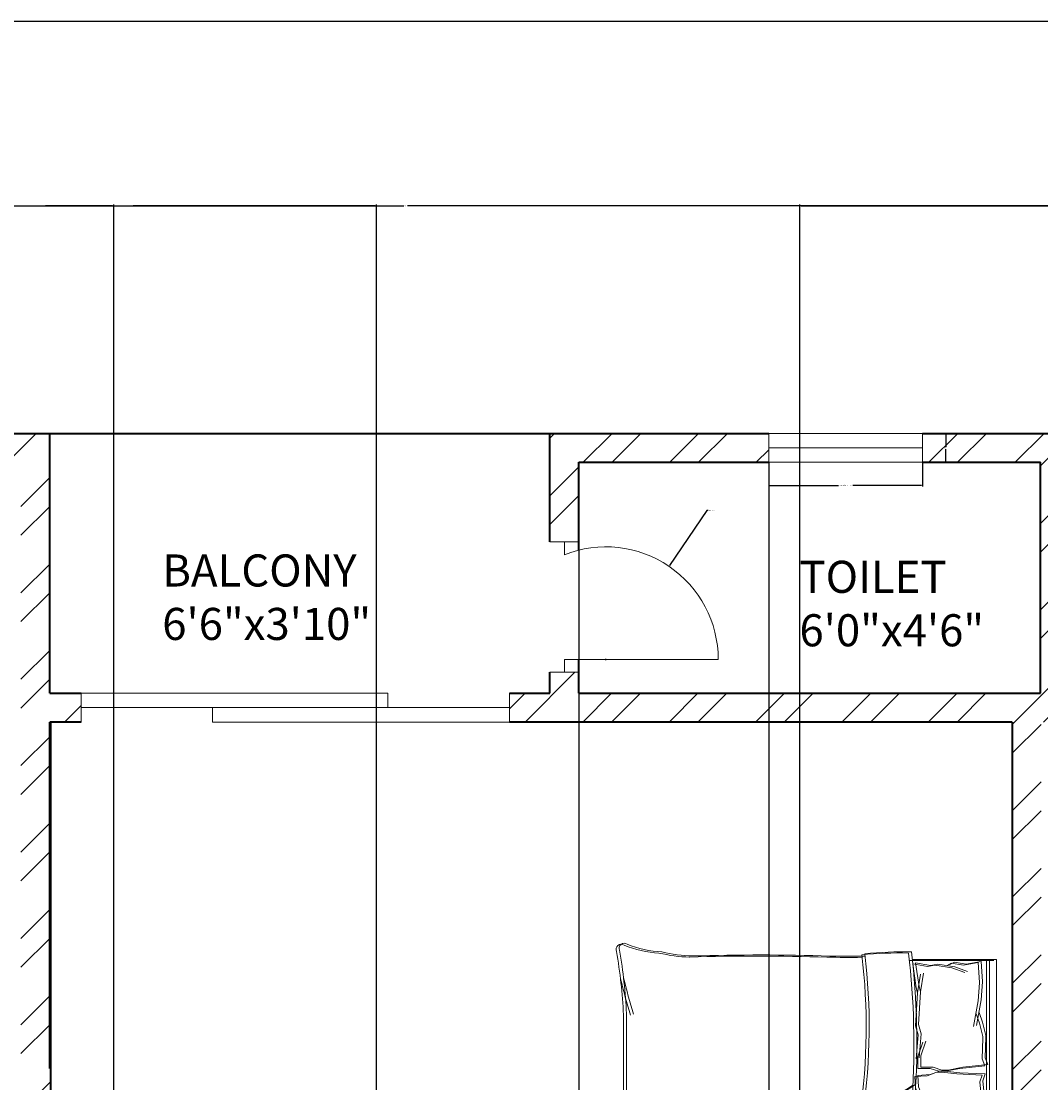
# Model space of a CAD drawing. Units: inches. Extents: x 2064 to 2782, y 1196 to 2299.
# Tile 8 of 11: x 2331 to 2490, y 2133 to 2299. Entities that reach past the tile are written whole.
import ezdxf

# ---------------------------------------------------------------- set-up
doc = ezdxf.new("R2010")
doc.units = ezdxf.units.IN
for name, color, linetype, lineweight in [('A-ANNO-DIMS', 2, 'Continuous', 18), ('A-ANNO-TTLB', 7, 'Continuous', 25), ('A-AREA-IDEN', 7, 'Continuous', 18), ('A-DOOR', 11, 'Continuous', 18), ('A-FURN', 8, 'Continuous', 13), ('A-GLAZ', 151, 'Continuous', 18), ('A-WALL', 7, 'Continuous', 35), ('A-WALL-PATT', 9, 'Continuous', 13)]:
    doc.layers.add(name, color=color, linetype=linetype, lineweight=lineweight)
doc.styles.get("Standard").update_dxf_attribs({"font": 'arial.ttf'})
doc.dimstyles.get("Standard").update_dxf_attribs({"dimtxt": 0.18, "dimasz": 0.18, "dimexe": 0.18, "dimexo": 0.0625, "dimgap": 0.09, "dimtad": 0, "dimtih": 1, "dimtoh": 1, "dimdec": 4, "dimzin": 0, "dimdsep": 46, "dimtxsty": 'Standard', "dimcen": 0.09, "dimadec": 0, "dimazin": 0, "dimtfac": 1, "dimtdec": 4, "dimtofl": 0, "dimtmove": 0, "dimatfit": 3, "dimfxl": 1, "dimtolj": 1, "dimtzin": 0, "dimarcsym": 0})

# ---------------------------------------------------------------- blocks, each defined once
blk = doc.blocks.new('BED-DOUBLE')
for p, q in [((2.53, 46.14), (2.53, 59.33)), ((2.53, 46.14), (2.53, 59.33)), ((2.53, 59.33), (37.35, 59.33)), ((2.53, 58.22), (37.35, 58.22)), ((2.53, 58.22), (37.35, 58.22)), ((2.7, 45.67), (2.7, 58.87)), ((2.7, 45.67), (2.7, 58.87)), ((17.88, 57.55), (18.93, 57.97)), ((17.88, 57.55), (18.93, 57.97)), ((18.93, 57.97), (19.35, 54.07)), ((18.93, 57.97), (19.35, 54.07)), ((37.35, 59.33), (37.35, 39.95)), ((37.35, 59.33), (37.35, 39.95)), ((37.52, 59.33), (37.52, 58.87)), ((37.52, 58.87), (37.52, 39.48)), ((37.52, 58.87), (37.52, 39.48)), ((2.7, 57.75), (37.52, 57.75)), ((2.7, 57.75), (37.52, 57.75)), ((2.84, 56.9), (5.96, 57.14)), ((2.84, 56.9), (5.96, 57.14)), ((2.84, 56.92), (3.26, 54.6)), ((2.84, 56.92), (3.26, 54.6)), ((3, 56.45), (3.43, 54.14)), ((3, 56.45), (3.43, 54.14)), ((3.01, 56.44), (6.13, 56.68)), ((3.01, 56.44), (6.13, 56.68)), ((5.96, 57.14), (6.04, 57.13)), ((5.96, 57.14), (6.04, 57.13)), ((6.04, 57.13), (8.82, 56.92)), ((6.04, 57.13), (8.82, 56.92)), ((6.13, 56.68), (6.2, 56.66)), ((6.13, 56.68), (6.2, 56.66)), ((6.2, 56.66), (8.99, 56.45)), ((6.2, 56.66), (8.99, 56.45)), ((8.82, 56.92), (12.82, 56.18)), ((8.82, 56.92), (12.82, 56.18)), ((8.99, 56.45), (12.99, 55.72)), ((8.99, 56.45), (12.99, 55.72)), ((10.82, 56.6), (12.3, 57.13)), ((10.82, 56.6), (12.3, 57.13)), ((10.99, 56.14), (12.46, 56.66)), ((10.99, 56.14), (12.46, 56.66)), ((12.3, 57.13), (14.4, 57.66)), ((12.3, 57.13), (14.4, 57.66)), ((12.46, 56.66), (14.57, 57.19)), ((12.46, 56.66), (14.57, 57.19)), ((14.4, 57.66), (14.64, 57.66)), ((14.4, 57.66), (14.64, 57.66)), ((14.57, 57.19), (14.8, 57.19)), ((14.57, 57.19), (14.8, 57.19)), ((14.64, 57.66), (17.88, 57.55)), ((14.64, 57.66), (17.88, 57.55)), ((14.8, 57.19), (18.04, 57.09)), ((14.8, 57.19), (18.04, 57.09)), ((18.04, 57.09), (19.1, 57.51)), ((18.04, 57.09), (19.1, 57.51)), ((19.1, 57.51), (19.52, 53.61)), ((19.1, 57.51), (19.52, 53.61)), ((20.38, 57.52), (20.2, 53.6)), ((20.38, 57.52), (20.21, 53.6)), ((20.55, 57.05), (20.37, 53.14)), ((20.55, 57.05), (20.37, 53.14)), ((21.46, 57.16), (20.38, 57.52)), ((21.46, 57.16), (20.38, 57.52)), ((21.63, 56.7), (20.55, 57.05)), ((21.63, 56.7), (20.55, 57.05)), ((24.69, 57.47), (21.46, 57.16)), ((24.69, 57.47), (21.46, 57.16)), ((24.85, 57.01), (21.63, 56.7)), ((24.85, 57.01), (21.63, 56.7)), ((24.92, 57.49), (24.69, 57.47)), ((24.92, 57.49), (24.69, 57.47)), ((25.09, 57.02), (24.85, 57.01)), ((25.09, 57.02), (24.85, 57.01)), ((27.05, 57.09), (24.92, 57.49)), ((27.05, 57.09), (24.92, 57.49)), ((27.22, 56.63), (25.09, 57.02)), ((27.22, 56.63), (25.09, 57.02)), ((30.54, 57.1), (26.59, 56.11)), ((30.54, 57.1), (26.59, 56.11)), ((30.7, 56.63), (26.75, 55.65)), ((30.7, 56.63), (26.75, 55.65)), ((28.56, 56.66), (27.05, 57.09)), ((28.56, 56.66), (27.05, 57.09)), ((28.73, 56.19), (27.22, 56.63)), ((28.73, 56.19), (27.22, 56.63)), ((33.3, 57.48), (30.54, 57.1)), ((33.3, 57.48), (30.54, 57.1)), ((33.47, 57.02), (30.7, 56.63)), ((33.47, 57.02), (30.7, 56.63)), ((36.51, 57.47), (32.57, 57.54)), ((32.57, 57.54), (33.3, 57.48)), ((36.51, 57.47), (32.57, 57.54)), ((32.57, 57.54), (33.3, 57.48)), ((36.68, 57.01), (32.74, 57.08)), ((32.74, 57.08), (33.47, 57.02)), ((36.67, 57.01), (32.74, 57.08)), ((32.74, 57.08), (33.47, 57.02)), ((36.51, 57.47), (36.23, 55.13)), ((36.51, 57.47), (36.23, 55.13)), ((36.68, 57.01), (36.4, 54.67)), ((36.67, 57.01), (36.4, 54.67)), ((3.68, 52.81), (4.42, 54.81)), ((3.68, 52.81), (4.42, 54.81)), ((35.92, 53.32), (35.06, 55.27)), ((35.92, 53.32), (35.06, 55.27)), ((36.09, 52.85), (35.23, 54.8)), ((36.09, 52.85), (35.23, 54.8)), ((36.23, 55.13), (36.67, 53.26)), ((36.23, 55.13), (36.67, 53.26)), ((36.4, 54.67), (36.83, 52.79)), ((36.4, 54.67), (36.83, 52.79)), ((3.26, 54.6), (2.94, 52.71)), ((3.26, 54.6), (2.94, 52.71)), ((3.43, 54.14), (3.11, 52.24)), ((3.43, 54.14), (3.11, 52.24)), ((3.85, 52.34), (4.58, 54.35)), ((3.85, 52.34), (4.58, 54.35)), ((19.35, 54.07), (19.77, 51.76)), ((19.35, 54.07), (19.77, 51.76)), ((19.52, 53.61), (19.94, 51.29)), ((19.52, 53.61), (19.94, 51.29)), ((20.21, 53.6), (19.93, 51.26)), ((20.2, 53.6), (19.93, 51.26)), ((20.37, 53.14), (20.1, 50.8)), ((20.37, 53.14), (20.1, 50.8)), ((36.51, 50.72), (35.92, 53.32)), ((36.51, 50.72), (35.92, 53.32)), ((36.67, 53.26), (36.29, 52.5)), ((36.67, 53.26), (36.29, 52.5)), ((2.94, 52.71), (3.36, 51.97)), ((2.94, 52.71), (3.36, 51.97)), ((3.11, 52.24), (3.53, 51.5)), ((3.11, 52.24), (3.53, 51.5)), ((3.26, 50.18), (3.68, 52.81)), ((3.26, 50.18), (3.68, 52.81)), ((3.43, 49.71), (3.85, 52.34)), ((3.43, 49.71), (3.85, 52.34)), ((19.77, 51.76), (19.77, 50.81)), ((19.77, 51.76), (19.77, 50.81)), ((36.68, 50.25), (36.09, 52.85)), ((36.67, 50.25), (36.09, 52.85)), ((36.83, 52.79), (36.46, 52.03)), ((36.83, 52.79), (36.46, 52.03)), ((3.47, 49.02), (3.26, 50.18)), ((3.47, 49.02), (3.26, 50.18)), ((3.64, 48.55), (3.43, 49.71)), ((3.64, 48.55), (3.43, 49.71)), ((19.77, 50.81), (19.35, 49.44)), ((19.77, 50.81), (19.35, 49.44)), ((19.94, 50.34), (19.52, 48.97)), ((19.94, 50.34), (19.52, 48.97)), ((19.93, 51.26), (19.99, 50.32)), ((19.93, 51.26), (19.99, 50.32)), ((19.94, 51.29), (19.94, 50.34)), ((19.94, 51.29), (19.94, 50.34)), ((19.99, 50.32), (20.49, 48.98)), ((19.99, 50.32), (20.49, 48.98)), ((20.1, 50.8), (20.15, 49.85)), ((20.1, 50.8), (20.15, 49.85)), ((20.15, 49.85), (20.66, 48.51)), ((20.15, 49.85), (20.66, 48.51)), ((36.37, 49.55), (36.51, 50.72)), ((36.37, 49.55), (36.51, 50.72)), ((36.54, 49.08), (36.68, 50.25)), ((36.54, 49.08), (36.67, 50.25)), ((3.05, 46.7), (3.47, 49.02)), ((3.05, 46.7), (3.47, 49.02)), ((3.21, 46.24), (3.64, 48.55)), ((3.21, 46.24), (3.64, 48.55)), ((17.56, 47.49), (15.27, 48.28)), ((17.56, 47.49), (15.27, 48.28)), ((19.35, 49.44), (19.35, 47.49)), ((19.35, 49.44), (19.35, 47.49)), ((19.52, 48.97), (19.52, 47.02)), ((19.52, 48.97), (19.52, 47.02)), ((20.49, 48.98), (20.62, 47.03)), ((20.49, 48.98), (20.62, 47.03)), ((20.66, 48.51), (20.78, 46.56)), ((20.66, 48.51), (20.78, 46.56)), ((22.4, 47.14), (24.64, 48.08)), ((22.4, 47.14), (24.64, 48.08)), ((36.94, 47.26), (36.37, 49.55)), ((36.94, 47.26), (36.37, 49.55)), ((37.1, 46.79), (36.54, 49.08)), ((37.1, 46.79), (36.54, 49.08)), ((6.76, 47.23), (3.05, 46.7)), ((6.76, 47.23), (3.05, 46.7)), ((6.93, 46.76), (3.21, 46.24)), ((6.93, 46.76), (3.21, 46.24)), ((4.65, 47.95), (7.59, 47.46)), ((4.65, 47.95), (7.59, 47.46)), ((4.82, 47.48), (7.75, 47)), ((4.82, 47.48), (7.75, 47)), ((7.59, 47.46), (6.76, 47.23)), ((7.59, 47.46), (6.76, 47.23)), ((7.75, 47), (6.93, 46.76)), ((7.75, 47), (6.93, 46.76)), ((7.59, 47.46), (12.69, 47.15)), ((7.59, 47.46), (12.69, 47.15)), ((7.75, 47), (12.86, 46.68)), ((7.75, 47), (12.86, 46.68)), ((12.69, 47.15), (14.12, 47.55)), ((12.69, 47.15), (14.12, 47.55)), ((12.86, 46.68), (14.29, 47.09)), ((12.86, 46.68), (14.29, 47.09)), ((14.12, 47.55), (17.86, 47.26)), ((14.12, 47.55), (17.86, 47.26)), ((14.29, 47.09), (18.03, 46.79)), ((14.29, 47.09), (18.03, 46.79)), ((17.73, 47.02), (15.44, 47.82)), ((17.73, 47.02), (15.44, 47.82)), ((19.35, 47.49), (17.56, 47.49)), ((19.35, 47.49), (17.56, 47.49)), ((19.52, 47.02), (17.73, 47.02)), ((19.52, 47.02), (17.73, 47.02)), ((20.62, 47.03), (22.4, 47.14)), ((20.62, 47.03), (22.4, 47.14)), ((20.78, 46.56), (22.57, 46.67)), ((20.78, 46.56), (22.57, 46.67)), ((22.05, 46.67), (25.1, 41.94)), ((22.05, 46.67), (25.1, 41.94)), ((22.57, 46.67), (24.81, 47.61)), ((22.57, 46.67), (24.81, 47.61)), ((29.61, 44.53), (23.54, 46.67)), ((29.61, 44.53), (23.54, 46.67)), ((23.72, 47.95), (26.66, 47.46)), ((23.72, 47.95), (26.66, 47.46)), ((23.89, 47.48), (26.83, 47)), ((23.89, 47.48), (26.83, 47)), ((26.66, 47.46), (31.77, 47.15)), ((26.66, 47.46), (31.77, 47.15)), ((26.83, 47), (31.94, 46.68)), ((26.83, 47), (31.94, 46.68)), ((31.77, 47.15), (33.2, 47.55)), ((31.77, 47.15), (33.2, 47.55)), ((31.94, 46.68), (33.36, 47.09)), ((31.94, 46.68), (33.36, 47.09)), ((33.2, 47.55), (36.94, 47.26)), ((33.2, 47.55), (36.94, 47.26)), ((33.36, 47.09), (37.1, 46.79)), ((33.36, 47.09), (37.1, 46.79)), ((22.21, 46.2), (25.26, 41.47)), ((22.21, 46.2), (25.26, 41.47)), ((29.78, 44.07), (23.7, 46.2)), ((29.78, 44.07), (23.7, 46.2)), ((33.67, 43.07), (29.61, 44.53)), ((33.67, 43.07), (29.61, 44.53)), ((33.84, 42.6), (29.78, 44.07)), ((33.84, 42.6), (29.78, 44.07)), ((35.82, 41.49), (33.67, 43.07)), ((35.82, 41.49), (33.67, 43.07)), ((25.1, 41.94), (26.34, 38.67)), ((25.1, 41.94), (26.34, 38.67)), ((25.26, 41.47), (26.51, 38.2)), ((25.26, 41.47), (26.51, 38.2)), ((35.98, 41.02), (33.84, 42.6)), ((35.98, 41.02), (33.84, 42.6)), ((38.52, 39.12), (35.82, 41.49)), ((38.52, 39.12), (35.82, 41.49)), ((38.68, 38.65), (35.98, 41.02)), ((38.68, 38.65), (35.98, 41.02)), ((26.34, 38.67), (26.56, 37.2)), ((26.34, 38.67), (26.56, 37.2)), ((26.51, 38.2), (26.73, 36.74)), ((26.51, 38.2), (26.73, 36.74)), ((28.37, 37.65), (29.84, 38.33)), ((28.37, 37.65), (29.84, 38.33)), ((29.84, 38.33), (32.32, 38.67)), ((29.84, 38.33), (32.32, 38.67)), ((30, 37.87), (32.49, 38.2)), ((30, 37.87), (32.49, 38.2)), ((32.32, 38.67), (35.14, 38.9)), ((32.32, 38.67), (35.14, 38.9)), ((32.49, 38.2), (35.31, 38.43)), ((32.49, 38.2), (35.31, 38.43)), ((35.14, 38.9), (37.4, 38.67)), ((35.14, 38.9), (37.4, 38.67)), ((35.31, 38.43), (37.56, 38.2)), ((35.31, 38.43), (37.56, 38.2)), ((37.4, 38.67), (38.52, 39.12)), ((37.4, 38.67), (38.52, 39.12)), ((37.56, 38.2), (38.68, 38.65)), ((37.56, 38.2), (38.68, 38.65)), ((38.57, 37.85), (38.52, 39.12, 2.82)), ((38.57, 37.85), (38.52, 39.12, 2.82)), ((38.74, 37.38), (38.68, 38.65, 2.82)), ((38.74, 37.38), (38.68, 38.65, 2.82)), ((26.56, 37.2), (28.37, 37.65)), ((26.56, 37.2), (28.37, 37.65)), ((26.73, 36.74), (28.54, 37.19)), ((26.73, 36.74), (28.54, 37.19)), ((28.54, 37.19), (30, 37.87)), ((28.54, 37.19), (30, 37.87)), ((10.97, 1.6), (28.91, 1.6)), ((10.97, 1.6), (28.91, 1.6)), ((11.14, 1.14), (29.07, 1.14)), ((11.14, 1.14), (29.07, 1.14))]:
    blk.add_line(p, q)
for centre, radius, start, end in [((15.56, -73.3), 120.19, 86.0865, 96.7821), ((15.56, -73.3), 120.19, 86.0865, 96.7821), ((15.73, -73.76), 120.19, 86.0865, 96.7821), ((15.73, -73.76), 120.19, 86.0865, 96.7821), ((62.04, 44.69), 60.69, 178.7218, 185.604), ((62.04, 44.69), 60.69, 178.7218, 185.604), ((62.21, 44.23), 60.69, 178.7218, 185.604), ((62.21, 44.23), 60.69, 178.7218, 185.604), ((12.94, -54.55), 94, 81.7845, 96.9006), ((12.94, -54.55), 94, 81.7845, 96.9006), ((13.1, -55.01), 94, 81.7845, 96.9006), ((13.1, -55.01), 94, 81.7845, 96.9006), ((-121.89, 36.62), 123.93, 358.4762, 1.0082), ((-121.89, 36.62), 123.93, 358.4762, 1.0082), ((-121.72, 36.16), 123.93, 358.4762, 1.0082), ((-121.72, 36.16), 123.93, 358.4762, 1.0082), ((31.87, 33.79), 4.53, 78.6608, 113.7384), ((31.87, 33.79), 4.53, 78.6608, 113.7384), ((37.39, 64.18), 26.36, 259.8763, 272.5657), ((37.39, 64.18), 26.36, 259.8763, 272.5657), ((26.69, 37.16), 0.134, 160.2464, 271.1377), ((26.69, 37.16), 0.134, 160.2464, 271.1377), ((22.7, 58.25), 21.6, 280.6617, 289.8806), ((22.7, 58.25), 21.6, 280.6617, 289.8806), ((26.86, 36.69), 0.134, 160.2464, 271.1377), ((26.86, 36.69), 0.134, 160.2464, 271.1377), ((22.86, 57.79), 21.6, 280.6617, 289.8806), ((22.86, 57.79), 21.6, 280.6617, 289.8806), ((32.04, 33.32), 4.53, 78.6608, 113.7384), ((32.04, 33.32), 4.53, 78.6608, 113.7384), ((37.56, 63.72), 26.36, 259.8763, 272.5657), ((37.56, 63.72), 26.36, 259.8763, 272.5657), ((132.79, 32.88), 94.35, 176.9791, 183.8365), ((132.79, 32.88), 94.35, 176.9791, 183.8365), ((132.95, 32.41), 94.35, 176.9791, 183.8365), ((132.95, 32.41), 94.35, 176.9791, 183.8365), ((353.21, 22.46), 351.38, 178.2277, 181.7185), ((353.21, 22.46), 351.38, 178.2277, 181.7185), ((353.38, 21.99), 351.38, 178.2277, 181.7185), ((353.38, 21.99), 351.38, 178.2277, 181.7185), ((-3284.8, 9.92), 3323.5, 0.00217, 0.28689), ((-3284.8, 9.92), 3323.5, 0.00217, 0.28689), ((-3284.64, 9.46), 3323.5, 0.00217, 0.28689), ((-3284.64, 9.46), 3323.5, 0.00217, 0.28689), ((-19.6, 12.33), 21.59, 346.0648, 358.9113), ((-19.6, 12.33), 21.59, 346.0648, 358.9113), ((-19.43, 11.87), 21.59, 346.0648, 358.9113), ((-19.43, 11.87), 21.59, 346.0648, 358.9113), ((55.48, 9.31), 16.8, 177.4714, 206.4681), ((55.48, 9.31), 16.8, 177.4714, 206.4681), ((55.65, 8.84), 16.8, 177.4714, 206.4681), ((55.65, 8.84), 16.8, 177.4714, 206.4681), ((-15.78, 8.14), 17.17, 337.9751, 356.652), ((-15.78, 8.14), 17.17, 337.9751, 356.652), ((-15.61, 7.67), 17.17, 337.9751, 356.652), ((-15.61, 7.67), 17.17, 337.9751, 356.652), ((0.79, 1.26), 0.793, 146.1736, 293.4781), ((0.79, 1.26), 0.793, 146.1736, 293.4781), ((-12.55, 76.61), 77.56, 283.3832, 287.7053), ((-12.55, 76.61), 77.56, 283.3832, 287.7053), ((-12.38, 76.14), 77.56, 283.3832, 287.7053), ((-12.38, 76.14), 77.56, 283.3832, 287.7053), ((39.64, 1.87), 0.803, 242.6588, 356.02), ((39.64, 1.87), 0.803, 242.6588, 356.02), ((0.96, 0.79), 0.793, 146.1736, 293.4781), ((0.96, 0.79), 0.793, 146.1736, 293.4781), ((15.61, -86.98), 88.71, 92.9958, 99.4091), ((15.61, -86.98), 88.71, 92.9958, 99.4091), ((15.78, -87.45), 88.71, 92.9958, 99.4091), ((15.78, -87.45), 88.71, 92.9958, 99.4091), ((29.98, -95.32), 96.92, 84.4998, 90.6351), ((29.98, -95.32), 96.92, 84.4998, 90.6351), ((30.15, -95.78), 96.92, 84.4998, 90.6351), ((30.15, -95.78), 96.92, 84.4998, 90.6351), ((39.81, 1.41), 0.803, 242.6588, 356.02), ((39.81, 1.41), 0.803, 242.6588, 356.02)]:
    blk.add_arc(centre, radius, start, end)
blk = doc.blocks.new('WIN-24IN')
for p, q in [((0, 0), (0, 4.5)), ((0, 4.5), (0, 2.25)), ((0, 4.5), (24, 4.5)), ((24, 2.25), (24, 4.5)), ((24, 4.5), (24, 0)), ((0, 2.25), (24, 2.25)), ((24, 0), (0, 0))]:
    blk.add_line(p, q)
blk = doc.blocks.new('*D14')
at = {"layer": 'A-ANNO-DIMS', "color": 0, "lineweight": -2, "transparency": 16777216}
for p, q in [((2447.29, 2229.73), (2447.29, 2226.01)), ((2471.29, 2229.73), (2471.29, 2226.01)), ((2447.47, 2226.19), (2458.17, 2226.19)), ((2471.11, 2226.19), (2460.41, 2226.19))]:
    blk.add_line(p, q, dxfattribs=at)
at = {"layer": 'A-ANNO-DIMS', "color": 0, "transparency": 16777216}
for points in [[(2447.47, 2226.22), (2447.47, 2226.16), (2447.29, 2226.19)], [(2471.11, 2226.22), (2471.11, 2226.16), (2471.29, 2226.19)]]:
    blk.add_solid(points, dxfattribs=at)
at = {"layer": 'Defpoints', "color": 0, "transparency": 16777216}
for p in [(2447.29, 2229.79), (2471.29, 2229.79), (2471.29, 2226.19)]:
    blk.add_point(p, dxfattribs=at)
at = {"layer": 'A-ANNO-DIMS', "color": 0, "transparency": 16777216, "insert": (2459.29, 2226.19), "char_height": 0.18, "attachment_point": 5}
blk.add_mtext('\\A1;WINDOW 24 TYP.', dxfattribs=at)
blk = doc.blocks.new('*D15')
at = {"layer": 'A-ANNO-DIMS', "color": 0, "lineweight": -2, "transparency": 16777216}
for p, q in [((2471.35, 2234.29), (2475.07, 2234.29)), ((2474.89, 2234.11), (2474.89, 2232.22)), ((2474.89, 2229.97), (2474.89, 2231.86)), ((2471.35, 2229.79), (2475.07, 2229.79))]:
    blk.add_line(p, q, dxfattribs=at)
at = {"layer": 'A-ANNO-DIMS', "color": 0, "transparency": 16777216}
for points in [[(2474.86, 2234.11), (2474.92, 2234.11), (2474.89, 2234.29)], [(2474.86, 2229.97), (2474.92, 2229.97), (2474.89, 2229.79)]]:
    blk.add_solid(points, dxfattribs=at)
at = {"layer": 'Defpoints', "color": 0, "transparency": 16777216}
for p in [(2471.29, 2234.29), (2474.89, 2234.29), (2471.29, 2229.79)]:
    blk.add_point(p, dxfattribs=at)
at = {"layer": 'A-ANNO-DIMS', "color": 0, "transparency": 16777216, "insert": (2474.89, 2232.04), "char_height": 0.18, "attachment_point": 5}
blk.add_mtext('\\A1;5 TYP.', dxfattribs=at)
blk = doc.blocks.new('*D22')
at = {"layer": 'A-ANNO-DIMS', "color": 0, "lineweight": -2, "transparency": 16777216}
for p, q in [((2128.17, 2234.35), (2128.17, 2269.97)), ((2128.35, 2269.79), (2390.38, 2269.79)), ((2652.99, 2269.79), (2390.96, 2269.79)), ((2653.17, 2234.35), (2653.17, 2269.97))]:
    blk.add_line(p, q, dxfattribs=at)
at = {"layer": 'A-ANNO-DIMS', "color": 0, "transparency": 16777216}
for points in [[(2128.35, 2269.82), (2128.35, 2269.76), (2128.17, 2269.79)], [(2652.99, 2269.82), (2652.99, 2269.76), (2653.17, 2269.79)]]:
    blk.add_solid(points, dxfattribs=at)
at = {"layer": 'Defpoints', "color": 0, "transparency": 16777216}
for p in [(2653.17, 2269.79), (2128.17, 2234.29), (2653.17, 2234.29)]:
    blk.add_point(p, dxfattribs=at)
at = {"layer": 'A-ANNO-DIMS', "color": 0, "transparency": 16777216, "insert": (2390.67, 2269.79), "char_height": 0.18, "attachment_point": 5}
blk.add_mtext('\\A1;525', dxfattribs=at)
blk = doc.blocks.new('*D23')
at = {"layer": 'A-ANNO-DIMS', "color": 0, "lineweight": -2, "transparency": 16777216}
for p, q in [((2653.23, 2234.29), (2688.85, 2234.29)), ((2688.67, 2234.11), (2688.67, 1937.72)), ((2688.67, 1640.97), (2688.67, 1937.36)), ((2452.23, 1640.79), (2688.85, 1640.79))]:
    blk.add_line(p, q, dxfattribs=at)
at = {"layer": 'A-ANNO-DIMS', "color": 0, "transparency": 16777216}
for points in [[(2688.64, 2234.11), (2688.7, 2234.11), (2688.67, 2234.29)], [(2688.64, 1640.97), (2688.7, 1640.97), (2688.67, 1640.79)]]:
    blk.add_solid(points, dxfattribs=at)
at = {"layer": 'Defpoints', "color": 0, "transparency": 16777216}
for p in [(2653.17, 2234.29), (2688.67, 2234.29), (2452.17, 1640.79)]:
    blk.add_point(p, dxfattribs=at)
at = {"layer": 'A-ANNO-DIMS', "color": 0, "transparency": 16777216, "insert": (2688.67, 1937.54), "char_height": 0.18, "attachment_point": 5}
blk.add_mtext('\\A1;593.5', dxfattribs=at)
blk = doc.blocks.new('*D27')
at = {"layer": 'A-ANNO-DIMS', "color": 0, "lineweight": -2, "transparency": 16777216}
for p, q in [((2452.17, 1640.85), (2452.17, 2269.97)), ((2452.35, 2269.79), (2493.09, 2269.79)), ((2534.61, 2269.79), (2493.87, 2269.79)), ((2534.79, 1643.35), (2534.79, 2269.97))]:
    blk.add_line(p, q, dxfattribs=at)
at = {"layer": 'A-ANNO-DIMS', "color": 0, "transparency": 16777216}
for points in [[(2452.35, 2269.82), (2452.35, 2269.76), (2452.17, 2269.79)], [(2534.61, 2269.82), (2534.61, 2269.76), (2534.79, 2269.79)]]:
    blk.add_solid(points, dxfattribs=at)
at = {"layer": 'Defpoints', "color": 0, "transparency": 16777216}
for p in [(2534.79, 2269.79), (2534.79, 1643.29), (2452.17, 1640.79)]:
    blk.add_point(p, dxfattribs=at)
at = {"layer": 'A-ANNO-DIMS', "color": 0, "transparency": 16777216, "insert": (2493.48, 2269.79), "char_height": 0.18, "attachment_point": 5}
blk.add_mtext('\\A1;82.62', dxfattribs=at)
blk = doc.blocks.new('*D35')
at = {"layer": 'A-ANNO-DIMS', "color": 0, "lineweight": -2, "transparency": 16777216}
for p, q in [((2309.4, 1932.85), (2309.4, 2269.97)), ((2309.58, 2269.79), (2347.37, 2269.79)), ((2385.94, 2269.79), (2348.16, 2269.79)), ((2386.12, 1856.35), (2386.12, 2269.97))]:
    blk.add_line(p, q, dxfattribs=at)
at = {"layer": 'A-ANNO-DIMS', "color": 0, "transparency": 16777216}
for points in [[(2309.58, 2269.82), (2309.58, 2269.76), (2309.4, 2269.79)], [(2385.94, 2269.82), (2385.94, 2269.76), (2386.12, 2269.79)]]:
    blk.add_solid(points, dxfattribs=at)
at = {"layer": 'Defpoints', "color": 0, "transparency": 16777216}
for p in [(2386.12, 2269.79), (2309.4, 1932.79), (2386.12, 1856.29)]:
    blk.add_point(p, dxfattribs=at)
at = {"layer": 'A-ANNO-DIMS', "color": 0, "transparency": 16777216, "insert": (2347.76, 2269.79), "char_height": 0.18, "attachment_point": 5}
blk.add_mtext('\\A1;76.72', dxfattribs=at)
blk = doc.blocks.new('*D39')
at = {"layer": 'A-ANNO-DIMS', "color": 0, "lineweight": -2, "transparency": 16777216}
for p, q in [((2322.95, 1645.35), (2322.95, 2269.97)), ((2323.13, 2269.79), (2333.59, 2269.79)), ((2344.97, 2269.79), (2334.51, 2269.79)), ((2345.15, 1645.35), (2345.15, 2269.97))]:
    blk.add_line(p, q, dxfattribs=at)
at = {"layer": 'A-ANNO-DIMS', "color": 0, "transparency": 16777216}
for points in [[(2323.13, 2269.82), (2323.13, 2269.76), (2322.95, 2269.79)], [(2344.97, 2269.82), (2344.97, 2269.76), (2345.15, 2269.79)]]:
    blk.add_solid(points, dxfattribs=at)
at = {"layer": 'Defpoints', "color": 0, "transparency": 16777216}
for p in [(2345.15, 2269.79), (2322.95, 1645.29), (2345.15, 1645.29)]:
    blk.add_point(p, dxfattribs=at)
at = {"layer": 'A-ANNO-DIMS', "color": 0, "transparency": 16777216, "insert": (2334.05, 2269.79), "char_height": 0.18, "attachment_point": 5}
blk.add_mtext('\\A1;22.194', dxfattribs=at)
blk = doc.blocks.new('*D41')
at = {"layer": 'A-ANNO-DIMS', "color": 0, "lineweight": -2, "transparency": 16777216}
for p, q in [((2417.67, 2229.73), (2417.67, 1539.01)), ((2447.29, 2229.73), (2447.29, 1539.01)), ((2417.85, 1539.19), (2432.08, 1539.19)), ((2447.11, 1539.19), (2432.87, 1539.19))]:
    blk.add_line(p, q, dxfattribs=at)
at = {"layer": 'A-ANNO-DIMS', "color": 0, "transparency": 16777216}
for points in [[(2417.85, 1539.22), (2417.85, 1539.16), (2417.67, 1539.19)], [(2447.11, 1539.22), (2447.11, 1539.16), (2447.29, 1539.19)]]:
    blk.add_solid(points, dxfattribs=at)
at = {"layer": 'Defpoints', "color": 0, "transparency": 16777216}
for p in [(2417.67, 2229.79), (2447.29, 2229.79), (2447.29, 1539.19)]:
    blk.add_point(p, dxfattribs=at)
at = {"layer": 'A-ANNO-DIMS', "color": 0, "transparency": 16777216, "insert": (2432.48, 1539.19), "char_height": 0.18, "attachment_point": 5}
blk.add_mtext('\\A1;29.62', dxfattribs=at)
blk = doc.blocks.new('*D51')
at = {"layer": 'A-ANNO-DIMS', "color": 0, "lineweight": -2, "transparency": 16777216}
for p, q in [((2437.66, 2222.28), (2431.84, 2213.72)), ((2437.84, 2222.28), (2437.66, 2222.28)), ((2421.78, 2199.06), (2421.96, 2199.06)), ((2421.87, 2198.97), (2421.87, 2199.15))]:
    blk.add_line(p, q, dxfattribs=at)
at = {"layer": 'A-ANNO-DIMS', "color": 0, "transparency": 16777216}
blk.add_solid([(2431.81, 2213.74), (2431.86, 2213.71), (2431.74, 2213.57)], dxfattribs=at)
at = {"layer": 'Defpoints', "color": 0, "transparency": 16777216}
for p in [(2431.74, 2213.57), (2421.87, 2199.06)]:
    blk.add_point(p, dxfattribs=at)
at = {"layer": 'A-ANNO-DIMS', "color": 0, "transparency": 16777216, "insert": (2438.39, 2222.28), "char_height": 0.18, "attachment_point": 5}
blk.add_mtext('\\A1;R17.547', dxfattribs=at)

msp = doc.modelspace()

# ---------------------------------------------------------------- hatches: boundary and pattern name
at = {"layer": 'A-WALL-PATT'}
h = msp.add_hatch(dxfattribs=at)
h.set_pattern_fill('ANSI32', color=256)
h.paths.add_polyline_path([(2489.7688, 2189.2917), (2574.5454, 2189.2917), (2574.5454, 2191.5417), (2574.5454, 2193.7917), (2570.6691, 2193.7917), (2570.6691, 2197.3052), (2568.4191, 2197.3052), (2566.1691, 2197.3052), (2566.1691, 2193.7917), (2494.1691, 2193.7917), (2494.1691, 2229.7917), (2523.2441, 2229.7917), (2523.2441, 2234.2917), (2471.2886, 2234.2917), (2471.2886, 2229.7917), (2489.6691, 2229.7917), (2489.6691, 2193.7917), (2417.6691, 2193.7917), (2417.6691, 2197.0632), (2415.4191, 2197.0632), (2413.1691, 2197.0632), (2413.1691, 2193.7917), (2406.8865, 2193.7917), (2406.8865, 2189.2917), (2485.2688, 2189.2917), (2485.2688, 2063.2917), (2369.1629, 2063.2917), (2369.1629, 2058.7917), (2386.1222, 2058.7917), (2386.1222, 1856.2917), (2382.1576, 1856.2917), (2382.1576, 1851.7917), (2394.9764, 1851.7917), (2394.9764, 1854.0417), (2394.9764, 1856.2917), (2390.6222, 1856.2917), (2390.6222, 2058.7917), (2485.2688, 2058.7917), (2493.762, 2058.7917), (2493.762, 2061.0417), (2493.762, 2063.2917), (2489.7688, 2063.2917)])
h.paths.add_polyline_path([(2447.2886, 2234.2917), (2413.1691, 2234.2917), (2413.1691, 2217.3799), (2417.6691, 2217.3799), (2417.6691, 2229.7917), (2447.2886, 2229.7917)], flags=17)
h.paths.add_polyline_path([(2570.6691, 2234.2917), (2547.2441, 2234.2917), (2547.2441, 2229.7917), (2566.1691, 2229.7917), (2566.1691, 2216.5615), (2570.6691, 2216.5615)], flags=17)
h.paths.add_polyline_path([(2653.1691, 2189.2917), (2653.1691, 2193.7917), (2640.8843, 2193.7917), (2640.8843, 2189.2917), (2648.6691, 2189.2917), (2648.6691, 2162.7138), (2653.1691, 2162.7138)])
h.paths.add_polyline_path([(2653.1691, 2102.7138), (2648.6691, 2102.7138), (2648.6691, 2063.2917), (2526.7281, 2063.2917), (2526.7281, 2058.7917), (2541.1691, 2058.7917), (2541.1691, 1993.2917), (2545.6691, 1993.2917), (2545.6691, 1997.7917), (2545.6691, 2058.7917), (2648.6691, 2058.7917), (2648.6691, 2050.1099), (2653.1691, 2050.1099)])
h.paths.add_polyline_path([(2600.6691, 1856.2917), (2493.4607, 1856.2917), (2493.4607, 1851.7917), (2596.1691, 1851.7917), (2596.1691, 1695.7917), (2594.0816, 1695.7917), (2594.0816, 1691.2917), (2614.7905, 1691.2917), (2614.7905, 1645.2917), (2536.7905, 1645.2917), (2536.7905, 1691.2917), (2539.332, 1691.2917), (2539.332, 1693.5417), (2539.332, 1695.7917), (2452.1691, 1695.7917), (2452.1691, 1851.7917), (2456.0775, 1851.7917), (2456.0775, 1856.2917), (2427.1536, 1856.2917), (2427.1536, 1851.7917), (2447.6691, 1851.7917), (2447.6691, 1695.7917), (2447.6691, 1645.2917), (2405.1469, 1645.2917), (2405.1469, 1640.7917), (2452.1691, 1640.7917), (2452.1691, 1645.2917), (2452.1691, 1691.2917), (2534.7905, 1691.2917), (2534.7905, 1645.2917), (2534.7905, 1643.2917), (2614.7905, 1643.2917), (2616.7905, 1643.2917), (2616.7905, 1691.2917), (2622.4029, 1691.2917), (2622.4029, 1693.7143), (2622.4029, 1695.7917), (2600.6691, 1695.7917), (2600.6691, 1779.7917), (2648.6691, 1779.7917), (2648.6691, 1695.7917), (2646.4029, 1695.7917), (2646.4029, 1691.2917), (2653.1691, 1691.2917), (2653.1691, 1906.3508), (2648.6691, 1906.3508), (2648.6691, 1856.2917), (2648.6691, 1784.2917), (2600.6691, 1784.2917)])
h.paths.add_polyline_path([(2322.9532, 1819.5181), (2320.7032, 1819.5181), (2318.4532, 1819.5181), (2318.4532, 1695.7917), (2242.7664, 1695.7917), (2242.7664, 1691.2917), (2318.4532, 1691.2917), (2318.4532, 1640.7917), (2322.9532, 1640.7917), (2345.1469, 1640.7917), (2345.1469, 1643.0417), (2345.1469, 1645.2917), (2322.9532, 1645.2917), (2322.9532, 1691.2917), (2322.9532, 1695.7917)])
h.paths.add_polyline_path([(2166.1825, 1691.2917), (2164.1825, 1691.2917), (2164.1825, 1643.2917), (2166.1825, 1643.2917), (2246.1825, 1643.2917), (2246.1825, 1645.2917), (2246.1825, 1691.2917), (2244.1825, 1691.2917), (2244.1825, 1645.2917), (2166.1825, 1645.2917)])
h.paths.add_polyline_path([(2309.404, 1932.7917), (2204.1691, 1932.7917), (2204.1691, 1960.0962), (2199.6691, 1960.0962), (2199.6691, 1932.7917), (2132.6691, 1932.7917), (2132.6691, 1951.0737), (2128.1691, 1951.0737), (2128.1691, 1910.0412), (2132.6691, 1910.0412), (2132.6691, 1928.2917), (2304.904, 1928.2917), (2304.904, 1856.2917), (2304.904, 1851.7917), (2318.4532, 1851.7917), (2318.4532, 1848.8308), (2322.9532, 1848.8308), (2322.9532, 1851.7917), (2347.7631, 1851.7917), (2347.7631, 1856.2917), (2309.404, 1856.2917)])
h.paths.add_polyline_path([(2132.6691, 2044.9092), (2130.4191, 2044.9092), (2128.1691, 2044.9092), (2128.1691, 1987.0737), (2132.6691, 1987.0737), (2132.6691, 2004.7917), (2199.6691, 2004.7917), (2204.1691, 2004.7917), (2204.1691, 2009.2917), (2132.6691, 2009.2917)])
h.paths.add_polyline_path([(2186.6691, 2195.9329), (2184.4191, 2195.9329), (2184.4191, 2195.8929), (2182.1691, 2195.9329), (2182.1691, 2193.7917), (2128.1691, 2193.7917), (2128.1691, 2181.4967), (2132.6691, 2181.4967), (2132.6691, 2182.7769), (2132.6691, 2189.2917), (2182.1691, 2189.2917), (2182.1691, 2135.2917), (2179.804, 2135.2917), (2179.804, 2130.7917), (2190.215, 2130.7917), (2190.215, 2133.0417), (2190.215, 2135.2917), (2186.6691, 2135.2917)])
h.paths.add_polyline_path([(2340.0628, 2189.2917), (2340.0628, 2191.5417), (2340.0628, 2193.7917), (2335.1691, 2193.7917), (2335.1691, 2234.2917), (2280.6746, 2234.2917), (2280.6746, 2229.7917), (2330.6691, 2229.7917), (2330.6691, 2193.7917), (2330.6691, 2135.2917), (2218.6309, 2135.2917), (2218.6309, 2130.7917), (2330.7688, 2130.7917), (2330.7688, 2008.4023), (2335.2688, 2008.4023), (2335.2688, 2058.7917), (2338.9208, 2058.7917), (2338.9208, 2061.0417), (2338.9208, 2063.2917), (2335.2688, 2063.2917), (2335.2688, 2189.2917)])
h.paths.add_polyline_path([(2220.6746, 2234.2917), (2182.1691, 2234.2917), (2182.1691, 2227.4187), (2186.6691, 2227.4187), (2186.6691, 2229.7917), (2220.6746, 2229.7917), (2220.6746, 2232.0417)])
h.paths.add_polyline_path([(2158.8146, 2135.2917), (2132.6691, 2135.2917), (2132.6691, 2157.4967), (2128.1691, 2157.4967), (2128.1691, 2104.9092), (2132.6691, 2104.9092), (2132.6691, 2130.7917), (2158.8146, 2130.7917), (2158.8146, 2133.0417)])
h.paths.add_polyline_path([(2396.0464, 2062.2045), (2434.8868, 2062.2045), (2434.8868, 2080.8619), (2396.0464, 2080.8619)], flags=24)
h.paths.add_polyline_path([(2196.1396, 1653.3449), (2232.023, 1653.3449), (2232.023, 1672.0022), (2196.1396, 1672.0022)], flags=25)

# ---------------------------------------------------------------- linework, layer by layer
at = {"layer": 'A-ANNO-TTLB'}
msp.add_lwpolyline([(2063.9994, 2298.574), (2782.0941, 2298.574), (2782.0941, 1490.6238), (2063.9994, 1490.6238)], close=True, dxfattribs=at)
at = {"layer": 'A-DOOR'}
for p, q in [((2413.1691, 2217.3799), (2417.6691, 2217.3799)), ((2417.6691, 2217.3799), (2415.4191, 2217.3799)), ((2415.4191, 2217.3799), (2415.4191, 2215.3799)), ((2415.4191, 2197.0632), (2415.4191, 2199.0632)), ((2415.4191, 2199.0632), (2439.4191, 2199.0632)), ((2413.1691, 2197.0632), (2417.6691, 2197.0632)), ((2417.6691, 2197.0632), (2415.4191, 2197.0632))]:
    msp.add_line(p, q, dxfattribs=at)
msp.add_arc((2421.8726, 2199.0632), 17.5465, 0, 111.579624, dxfattribs=at)
at = {"layer": 'A-GLAZ'}
for p, q in [((2340.0628, 2193.7917), (2340.0628, 2189.2917)), ((2340.0628, 2193.7917), (2387.8929, 2193.7917)), ((2387.8929, 2193.7917), (2387.8929, 2191.5417)), ((2406.8865, 2191.5417), (2406.8865, 2193.7917)), ((2406.8865, 2193.7917), (2406.8865, 2189.2917)), ((2340.0628, 2189.2917), (2340.0628, 2191.5417)), ((2340.0628, 2191.5417), (2406.8865, 2191.5417)), ((2360.5373, 2191.5417), (2360.5373, 2189.2917)), ((2406.8865, 2189.2917), (2360.5373, 2189.2917))]:
    msp.add_line(p, q, dxfattribs=at)
at = {"layer": 'A-WALL'}
for p, q in [((2280.6746, 2234.2917), (2447.2886, 2234.2917)), ((2335.1691, 2193.7917), (2335.1691, 2234.2917)), ((2413.1691, 2217.3799), (2413.1691, 2234.2917)), ((2471.2886, 2234.2917), (2523.2441, 2234.2917)), ((2335.1691, 2193.7917), (2335.1691, 2229.7917)), ((2413.1691, 2217.3799), (2413.1691, 2229.7917)), ((2417.6691, 2229.7917), (2447.2886, 2229.7917)), ((2417.6691, 2216.0988), (2417.6691, 2229.7917)), ((2417.6691, 2216.0988), (2417.6691, 2229.7917)), ((2471.2886, 2229.7917), (2489.6691, 2229.7917)), ((2489.6691, 2193.7917), (2489.6691, 2229.7917)), ((2417.6691, 2193.7917), (2417.6691, 2199.0632)), ((2417.6691, 2193.7917), (2417.6691, 2199.0632)), ((2413.1691, 2193.7917), (2413.1691, 2197.0632)), ((2413.1691, 2193.7917), (2413.1691, 2197.0632)), ((2335.1691, 2193.7917), (2340.0628, 2193.7917)), ((2406.8865, 2193.7917), (2413.1691, 2193.7917)), ((2417.6691, 2193.7917), (2489.6691, 2193.7917)), ((2335.1691, 2135.2917), (2335.1691, 2189.2917)), ((2340.0628, 2189.2917), (2335.1691, 2189.2917)), ((2335.2688, 2189.2917), (2335.2688, 2063.2917)), ((2485.2688, 2189.2917), (2406.8865, 2189.2917)), ((2485.2688, 2189.2917), (2485.2688, 2063.2917))]:
    msp.add_line(p, q, dxfattribs=at)

# ---------------------------------------------------------------- block references
at = {"layer": 'A-FURN', "rotation": 269.9999998331855}
msp.add_blockref('BED-DOUBLE', (2423.5043, 2154.8008), dxfattribs=at)
at = {"layer": 'A-GLAZ'}
msp.add_blockref('WIN-24IN', (2447.2886, 2229.7917), dxfattribs=at)

# ---------------------------------------------------------------- texts
at = {"layer": 'A-AREA-IDEN', "char_height": 5, "attachment_point": 1}
for s, width, insert in [('BALCONY\\P6\'6"x3\'10"', 144.41847, (2352.7081, 2215.4272)), ('TOILET\\P6\'0"x4\'6"', 73.599498, (2452.0841, 2214.4384))]:
    msp.add_mtext_dynamic_manual_height_columns(s, width=width, gutter_width=12.5, heights=[0], dxfattribs=dict(at, insert=insert))

# ---------------------------------------------------------------- dimensions: what is measured, and where the dimension line sits
at = {"layer": 'A-ANNO-DIMS'}
for base, p1, p2, override, picture, middle in [((2653.1691, 2269.7917), (2128.1691, 2234.2917), (2653.1691, 2234.2917), {"dimdec": 0, "dimlfac": 1, "dimrnd": 0, "dimzin": 0, "dimdsep": 46, "dimlunit": 2}, '*D22', (2390.6691, 2269.7917)), ((2386.1222, 2269.7917), (2309.404, 1932.7917), (2386.1222, 1856.2917), {"dimdec": 2, "dimlfac": 1, "dimrnd": 0, "dimzin": 0, "dimdsep": 46, "dimlunit": 2}, '*D35', (2347.7631, 2269.7917)), ((2345.1469, 2269.7917), (2322.9532, 1645.2917), (2345.1469, 1645.2917), {"dimdec": 3, "dimlfac": 1, "dimrnd": 0, "dimzin": 0, "dimdsep": 46, "dimlunit": 2}, '*D39', (2334.0501, 2269.7917)), ((2534.7905, 2269.7917), (2452.1691, 1640.7917), (2534.7905, 1643.2917), {"dimdec": 2, "dimlfac": 1, "dimrnd": 0, "dimzin": 0, "dimdsep": 46, "dimlunit": 2}, '*D27', (2493.4798, 2269.7917)), ((2447.2886, 1539.1896), (2417.6691, 2229.7917), (2447.2886, 2229.7917), {"dimdec": 2, "dimlfac": 1, "dimrnd": 0, "dimzin": 0, "dimdsep": 46, "dimlunit": 2}, '*D41', (2432.4788, 1539.1896))]:
    dim = msp.add_linear_dim(base=base, p1=p1, p2=p2, dimstyle='Standard', override=override, dxfattribs=at)
    dim.commit()
    dim.dimension.update_dxf_attribs({"geometry": picture, "text_midpoint": middle})
dim = msp.add_linear_dim(base=(2688.6691, 2234.2917), p1=(2452.1691, 1640.7917), p2=(2653.1691, 2234.2917), angle=90, dimstyle='Standard', override={"dimdec": 1, "dimlfac": 1, "dimrnd": 0, "dimzin": 0, "dimdsep": 46, "dimlunit": 2}, dxfattribs=at)
dim.commit()
dim.dimension.update_dxf_attribs({"geometry": '*D23', "text_midpoint": (2688.6691, 1937.5417)})
dim = msp.add_linear_dim(base=(2474.8885528929, 2234.2916736115), p1=(2471.2885528929, 2229.7916736115), p2=(2471.2885528929, 2234.2916736115), angle=90, text='<> TYP.', dimstyle='Standard', override={"dimdec": 0, "dimlfac": 1, "dimrnd": 0, "dimzin": 0, "dimdsep": 46, "dimlunit": 2}, dxfattribs=at)
dim.commit()
dim.dimension.update_dxf_attribs({"geometry": '*D15', "text_midpoint": (2474.8885528929, 2232.0416736115)})
dim = msp.add_linear_dim(base=(2471.2886, 2226.1917), p1=(2447.2886, 2229.7917), p2=(2471.2886, 2229.7917), text='WINDOW <> TYP.', dimstyle='Standard', override={"dimdec": 0, "dimlfac": 1, "dimrnd": 0, "dimzin": 0, "dimdsep": 46, "dimlunit": 2}, dxfattribs=at)
dim.commit()
dim.dimension.update_dxf_attribs({"geometry": '*D14', "text_midpoint": (2459.2886, 2226.1917)})
dim = msp.add_radius_dim(center=(2421.8726, 2199.0632), mpoint=(2431.7379, 2213.5738), dimstyle='Standard', override={"dimdec": 3, "dimlfac": 1, "dimrnd": 0, "dimzin": 0, "dimdsep": 46, "dimlunit": 2}, dxfattribs=at)
dim.commit()
dim.dimension.update_dxf_attribs({"geometry": '*D51', "text_midpoint": (2438.3868, 2222.2801), "dimtype": 164})

doc.saveas('drawing.dxf')
